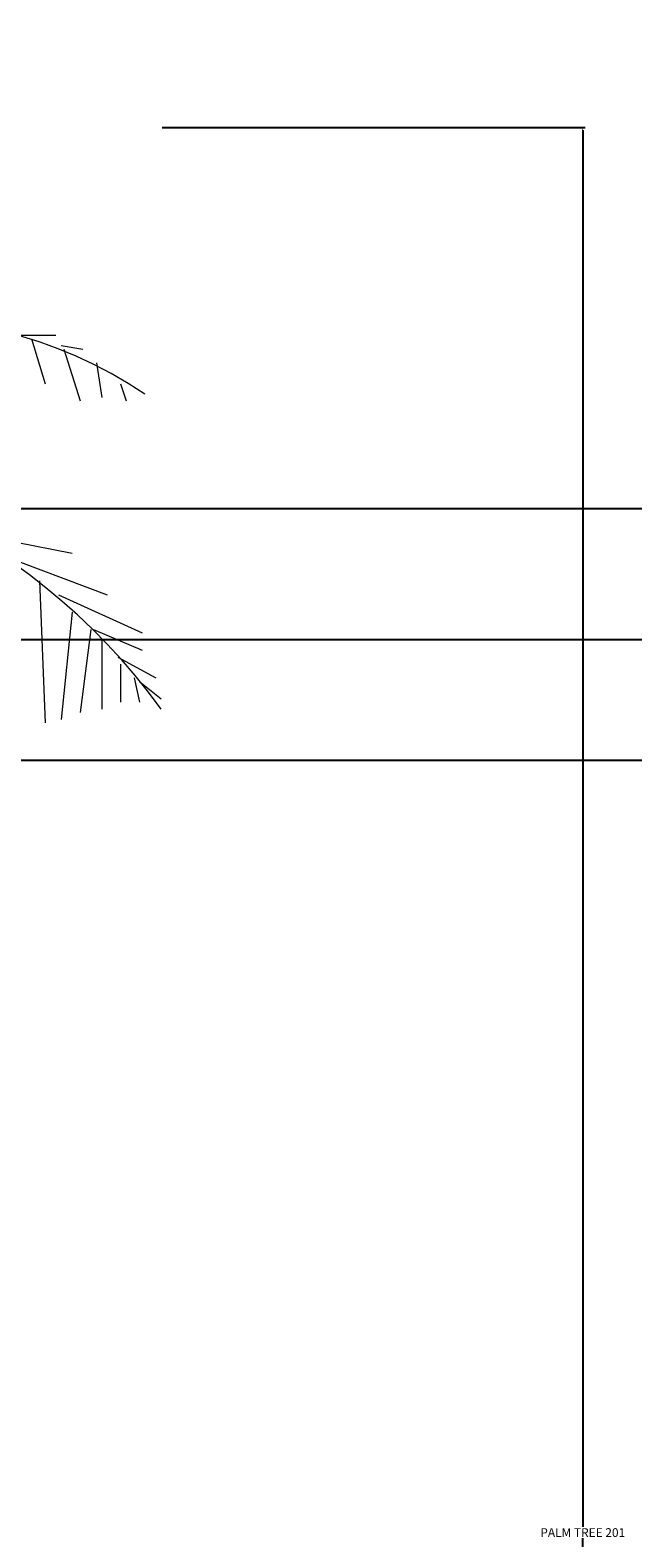
# Model space of a CAD drawing. Units: inches. Extents: x -13 to 809, y 112 to 656.
# Tile 49 of 55: x 702 to 746, y 251 to 359. Entities that reach past the tile are written whole.
import ezdxf

# ---------------------------------------------------------------- set-up
doc = ezdxf.new("R2010")
doc.units = ezdxf.units.IN
doc.header["$MEASUREMENT"] = 0
doc.layers.add('A-ANNO-DIMS', color=2, linetype='Continuous', lineweight=18)
doc.layers.add('L-PLNT', color=3, linetype='Continuous', lineweight=18)
doc.styles.get("Standard").update_dxf_attribs({"font": 'arial.ttf'})
doc.dimstyles.get("Standard").update_dxf_attribs({"dimtxt": 0.625, "dimasz": 0.18, "dimexe": 0.18, "dimexo": 0.0625, "dimgap": 0.09, "dimtad": 0, "dimtih": 1, "dimtoh": 1, "dimdec": 4, "dimzin": 0, "dimdsep": 46, "dimlunit": 4, "dimtxsty": 'Standard', "dimcen": 0.09, "dimadec": 0, "dimazin": 0, "dimtfac": 1, "dimtdec": 4, "dimtofl": 0, "dimtmove": 0, "dimatfit": 3, "dimfxl": 1, "dimtolj": 1, "dimtzin": 0, "dimarcsym": 0})

# ---------------------------------------------------------------- blocks, each defined once
blk = doc.blocks.new('Tree - palm elevation')
for p, q in [((32.512, 186.299), (35.218, 186.299)), ((33.479, 186.051), (34.445, 182.83)), ((35.605, 185.556), (37.151, 185.308)), ((35.798, 185.308), (36.958, 181.591)), ((38.118, 184.317), (38.504, 181.838)), ((39.857, 182.83), (40.244, 181.591)), ((28.839, 172.174), (36.378, 170.687)), ((30.966, 170.687), (38.891, 167.713)), ((34.058, 168.705), (34.445, 158.545)), ((35.412, 167.713), (41.404, 164.988)), ((36.378, 166.474), (35.605, 158.792)), ((37.731, 165.235), (36.958, 159.288)), ((37.924, 165.235), (41.404, 163.749)), ((38.504, 164.492), (38.504, 159.536)), ((39.664, 163.253), (42.37, 161.766)), ((39.857, 162.757), (39.857, 160.031)), ((40.824, 161.766), (41.21, 160.031)), ((41.21, 161.518), (42.757, 160.279))]:
    blk.add_line(p, q)
for centre, radius, start, end in [((23.687, 155.341), 32.188, 56.19272, 134.3213), ((5.828, 132.718), 45.639, 35.98777, 95.82273)]:
    blk.add_arc(centre, radius, start, end)
blk = doc.blocks.new('*D9')
at = {"layer": 'A-ANNO-DIMS', "color": 0, "lineweight": -2, "transparency": 16777216}
for p, q in [((711.81, 351.8), (742.1, 351.8)), ((741.92, 351.62), (741.92, 251.63)), ((741.92, 150.81), (741.92, 250.81)), ((711.81, 150.63), (742.1, 150.63))]:
    blk.add_line(p, q, dxfattribs=at)
at = {"layer": 'A-ANNO-DIMS', "color": 0, "transparency": 16777216}
for points in [[(741.89, 351.62), (741.95, 351.62), (741.92, 351.8)], [(741.89, 150.81), (741.95, 150.81), (741.92, 150.63)]]:
    blk.add_solid(points, dxfattribs=at)
at = {"layer": 'Defpoints', "color": 0, "transparency": 16777216}
for p in [(711.75, 351.8), (741.92, 351.8), (711.75, 150.63)]:
    blk.add_point(p, dxfattribs=at)
at = {"layer": 'A-ANNO-DIMS', "color": 0, "transparency": 16777216, "insert": (741.92, 251.22), "char_height": 0.625, "attachment_point": 5}
blk.add_mtext('\\A1;PALM TREE 201', dxfattribs=at)
blk = doc.blocks.new('*D31')
at = {"layer": 'A-ANNO-DIMS', "color": 0, "lineweight": -2, "transparency": 16777216}
for p, q in [((621.07, 617.78), (807.77, 617.78)), ((807.59, 617.6), (807.59, 384.56)), ((807.59, 150.7), (807.59, 383.74)), ((621.07, 150.52), (807.77, 150.52))]:
    blk.add_line(p, q, dxfattribs=at)
at = {"layer": 'A-ANNO-DIMS', "color": 0, "transparency": 16777216}
for points in [[(807.56, 617.6), (807.62, 617.6), (807.59, 617.78)], [(807.56, 150.7), (807.62, 150.7), (807.59, 150.52)]]:
    blk.add_solid(points, dxfattribs=at)
at = {"layer": 'Defpoints', "color": 0, "transparency": 16777216}
for p in [(621.01, 617.78), (807.59, 617.78), (621.01, 150.52)]:
    blk.add_point(p, dxfattribs=at)
at = {"layer": 'A-ANNO-DIMS', "color": 0, "transparency": 16777216, "insert": (807.59, 384.15), "char_height": 0.625, "attachment_point": 5}
blk.add_mtext('\\A1;467.3', dxfattribs=at)
blk = doc.blocks.new('*D46')
at = {"layer": 'A-ANNO-DIMS', "color": 0, "lineweight": -2, "transparency": 16777216}
for p, q in [((160.98, 408.79), (807.77, 408.79)), ((807.59, 408.61), (807.59, 367.07)), ((807.59, 324.7), (807.59, 366.25)), ((160.98, 324.52), (807.77, 324.52))]:
    blk.add_line(p, q, dxfattribs=at)
at = {"layer": 'A-ANNO-DIMS', "color": 0, "transparency": 16777216}
for points in [[(807.56, 408.61), (807.62, 408.61), (807.59, 408.79)], [(807.56, 324.7), (807.62, 324.7), (807.59, 324.52)]]:
    blk.add_solid(points, dxfattribs=at)
at = {"layer": 'Defpoints', "color": 0, "transparency": 16777216}
for p in [(160.92, 408.79), (807.59, 408.79), (160.92, 324.52)]:
    blk.add_point(p, dxfattribs=at)
at = {"layer": 'A-ANNO-DIMS', "color": 0, "transparency": 16777216, "insert": (807.59, 366.66), "char_height": 0.625, "attachment_point": 5}
blk.add_mtext('\\A1;84.27', dxfattribs=at)
blk = doc.blocks.new('*D48')
at = {"layer": 'A-ANNO-DIMS', "color": 0, "lineweight": -2, "transparency": 16777216}
for p, q in [((319.57, 444.52), (807.77, 444.52)), ((807.59, 444.34), (807.59, 384.93)), ((807.59, 324.7), (807.59, 384.11)), ((319.57, 324.52), (807.77, 324.52))]:
    blk.add_line(p, q, dxfattribs=at)
at = {"layer": 'A-ANNO-DIMS', "color": 0, "transparency": 16777216}
for points in [[(807.56, 444.34), (807.62, 444.34), (807.59, 444.52)], [(807.56, 324.7), (807.62, 324.7), (807.59, 324.52)]]:
    blk.add_solid(points, dxfattribs=at)
at = {"layer": 'Defpoints', "color": 0, "transparency": 16777216}
for p in [(319.51, 444.52), (807.59, 444.52), (319.51, 324.52)]:
    blk.add_point(p, dxfattribs=at)
at = {"layer": 'A-ANNO-DIMS', "color": 0, "transparency": 16777216, "insert": (807.59, 384.52), "char_height": 0.625, "attachment_point": 5}
blk.add_mtext('\\A1;120', dxfattribs=at)
blk = doc.blocks.new('*D106')
at = {"layer": 'A-ANNO-DIMS', "color": 0, "lineweight": -2, "transparency": 16777216}
for p, q in [((319.57, 315.14), (807.77, 315.14)), ((807.59, 314.96), (807.59, 311.24)), ((807.59, 306.7), (807.59, 310.42)), ((337.57, 306.52), (807.77, 306.52))]:
    blk.add_line(p, q, dxfattribs=at)
at = {"layer": 'A-ANNO-DIMS', "color": 0, "transparency": 16777216}
for points in [[(807.56, 314.96), (807.62, 314.96), (807.59, 315.14)], [(807.56, 306.7), (807.62, 306.7), (807.59, 306.52)]]:
    blk.add_solid(points, dxfattribs=at)
at = {"layer": 'Defpoints', "color": 0, "transparency": 16777216}
for p in [(319.51, 315.14), (807.59, 315.14), (337.51, 306.52)]:
    blk.add_point(p, dxfattribs=at)
at = {"layer": 'A-ANNO-DIMS', "color": 0, "transparency": 16777216, "insert": (807.59, 310.83), "char_height": 0.625, "attachment_point": 5}
blk.add_mtext('\\A1;8.624', dxfattribs=at)

msp = doc.modelspace()

# ---------------------------------------------------------------- block references
at = {"layer": 'L-PLNT'}
msp.add_blockref('Tree - palm elevation', (668.9925, 150.6343), dxfattribs=at)

# ---------------------------------------------------------------- dimensions: what is measured, and where the dimension line sits
at = {"layer": 'A-ANNO-DIMS'}
for base, p1, p2, override, picture, middle in [((807.5888, 617.7828), (621.008, 150.5199), (621.008, 617.7828), {"dimdec": 1, "dimlfac": 1, "dimrnd": 0, "dimzin": 0, "dimdsep": 46, "dimlunit": 2}, '*D31', (807.5888, 384.1514)), ((807.5888, 444.5199), (319.5074, 324.5199), (319.5074, 444.5199), {"dimdec": 0, "dimlfac": 1, "dimrnd": 0, "dimzin": 0, "dimdsep": 46, "dimlunit": 2}, '*D48', (807.5888, 384.5199)), ((807.5888, 408.7939), (160.9184, 324.5199), (160.9184, 408.7939), {"dimdec": 2, "dimlfac": 1, "dimrnd": 0, "dimzin": 0, "dimdsep": 46, "dimlunit": 2}, '*D46', (807.5888, 366.6569)), ((807.5888, 315.1435), (337.5074, 306.5199), (319.5074, 315.1435), {"dimdec": 3, "dimlfac": 1, "dimrnd": 0, "dimzin": 0, "dimdsep": 46, "dimlunit": 2}, '*D106', (807.5888, 310.8317))]:
    dim = msp.add_linear_dim(base=base, p1=p1, p2=p2, angle=90, dimstyle='Standard', override=override, dxfattribs=at)
    dim.commit()
    dim.dimension.update_dxf_attribs({"geometry": picture, "text_midpoint": middle})
dim = msp.add_linear_dim(base=(741.9246, 351.8013), p1=(711.7495, 150.6343), p2=(711.7495, 351.8013), angle=90, text='PALM TREE <>', dimstyle='Standard', override={"dimdec": 0, "dimlfac": 1, "dimrnd": 0, "dimzin": 0, "dimdsep": 46, "dimlunit": 2}, dxfattribs=at)
dim.commit()
dim.dimension.update_dxf_attribs({"geometry": '*D9', "text_midpoint": (741.9246, 251.2178)})

doc.saveas('drawing.dxf')
